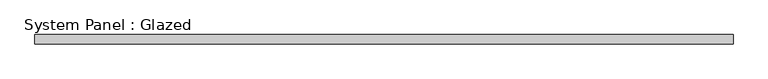
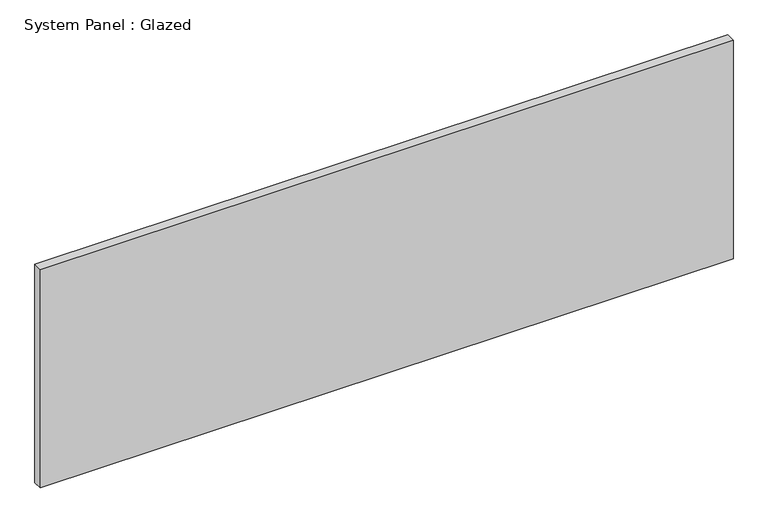
"""IFC4 building model written with IfcOpenShell, lengths in millimetres: plate geometry, System Panel : Glazed."""

from ifc_helpers import new_model, si_unit, origin, origin_with_axes, place, context, project, spatial, polyline, outline, extrude, source, transform, mapped, element, save


def system_panel_glazed_2daceabd(model_context):
    return source(origin(), model_context, "Body", "SweptSolid", [
        extrude(outline(polyline([(915.0000002, 24.5), (-915.0000002, 24.5), (-915.0000002, 49.5), (915.0000002, 49.5), (915.0000002, 24.5)])), origin_with_axes(), (0.0, 0.0, 1.0), 609.6),
    ])


if __name__ == "__main__":
    model = new_model("IFC4")
    model_context = context("Model", 3, world=origin())
    ifc_project = project(units=[si_unit("LENGTHUNIT", "METRE", prefix="MILLI")], contexts=[model_context])
    site = spatial("IfcSite", under=ifc_project)
    building = spatial("IfcBuilding", under=site)
    placement = place(None, origin())
    system_panel_glazed_shape = system_panel_glazed_2daceabd(model_context)
    element("IfcPlate", 1, ObjectType="System Panel : Glazed", at=placement, inside=building, context=model_context, shape_type="MappedRepresentation", body=[
        mapped(system_panel_glazed_shape, transform((0.0, 0.0, 0.0), x_axis=(1.0, 0.0, 0.0), y_axis=(0.0, 1.0, 0.0), z_axis=(0.0, 0.0, 1.0))),
    ])
    save(model, "model.ifc")

# Revit data of these elements
# Type "System Panel : Glazed"
#   Keynote = "H11"
#   Construction Type Id = "GSP4R"
#   Analytic Construction = "1/8 in Pilkington single glazing"
#   Visual Light Transmittance = 0.9
#   Solar Heat Gain Coefficient = 0.86
#   Heat Transfer Coefficient (U) = 6.7069 W/(m²·K)
#   Define Thermal Properties by = 1
# Element 1 (IfcPlate, "System Panel : Glazed")
#   Materials on its faces: "Glass"
# Materials
#   "Glass": class "Glass", colour RGB 0 128 192, transparency 0.9, Description = "Soda Lime Glass", Cost = 0
